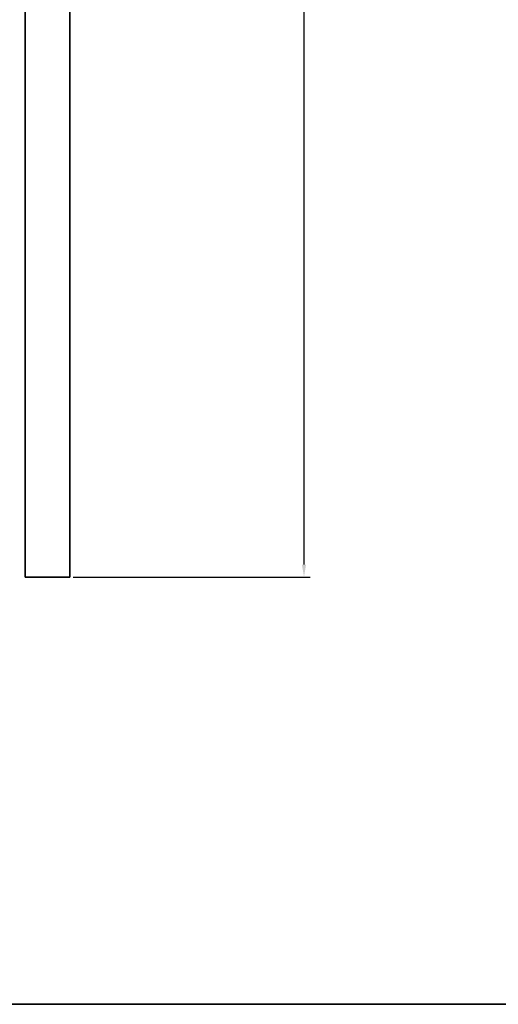
# Model space of a CAD drawing. Units: inches. Extents: x 1863 to 2938, y 1238 to 2492.
# Tile 5 of 12: x 2285 to 2381, y 1253 to 1452. Entities that reach past the tile are written whole.
import ezdxf

# ---------------------------------------------------------------- set-up
doc = ezdxf.new("R2010")
doc.units = ezdxf.units.IN
for name, color, linetype, lineweight in [('A-ANNO-DIMS', 2, 'Continuous', 18), ('A-ANNO-TTLB', 7, 'Continuous', 35), ('A-WALL', 7, 'Continuous', 35)]:
    doc.layers.add(name, color=color, linetype=linetype, lineweight=lineweight)
doc.styles.get("Standard").update_dxf_attribs({"font": 'arial.ttf'})
doc.dimstyles.new('ISO-25', dxfattribs={"dimtxt": 7, "dimasz": 2.5, "dimexe": 1.25, "dimexo": 0.625, "dimtad": 1, "dimdec": 0, "dimlunit": 3, "dimtxsty": 'Standard', "dimcen": 2.5, "dimadec": 0, "dimazin": 0, "dimtfac": 1, "dimtdec": 0, "dimtmove": 0, "dimatfit": 3, "dimfxl": 1, "dimarcsym": 0})

# ---------------------------------------------------------------- blocks, each defined once
blk = doc.blocks.new('*D3')
at = {"layer": 'A-ANNO-DIMS', "color": 0, "lineweight": -2, "transparency": 16777216}
for p, q in [((2295.26, 2076.56), (2343.03, 2076.56)), ((2341.78, 2074.06), (2341.78, 1342.06)), ((2295.26, 1339.56), (2343.03, 1339.56))]:
    blk.add_line(p, q, dxfattribs=at)
at = {"layer": 'A-ANNO-DIMS', "color": 0, "transparency": 16777216}
for points in [[(2341.36, 2074.06), (2342.2, 2074.06), (2341.78, 2076.56)], [(2341.36, 1342.06), (2342.2, 1342.06), (2341.78, 1339.56)]]:
    blk.add_solid(points, dxfattribs=at)
at = {"layer": 'Defpoints', "color": 0, "transparency": 16777216}
for p in [(2294.64, 2076.56), (2294.64, 1339.56), (2341.78, 1339.56)]:
    blk.add_point(p, dxfattribs=at)
at = {"layer": 'A-ANNO-DIMS', "color": 0, "transparency": 16777216, "insert": (2337.58, 1708.06), "char_height": 7, "attachment_point": 5, "rotation": 90}
blk.add_mtext('61\'-5"', dxfattribs=at)

msp = doc.modelspace()

# ---------------------------------------------------------------- linework, layer by layer
at = {"layer": 'A-ANNO-TTLB'}
msp.add_lwpolyline([(1863.2, 2492.19), (2938.41, 2492.19), (2938.41, 1253.47), (1863.2, 1253.47)], close=True, dxfattribs=at)
at = {"layer": 'A-WALL'}
for p, q in [((2285.64, 1339.56), (2285.64, 1495.56)), ((2294.64, 1495.56), (2294.64, 1339.56)), ((2294.64, 1339.56), (2285.64, 1339.56))]:
    msp.add_line(p, q, dxfattribs=at)

# ---------------------------------------------------------------- dimensions: what is measured, and where the dimension line sits
at = {"layer": 'A-ANNO-DIMS'}
dim = msp.add_linear_dim(base=(2341.78, 1339.56), p1=(2294.64, 2076.56), p2=(2294.64, 1339.56), angle=90, dimstyle='ISO-25', override={"dimclrd": 0, "dimclre": 0, "dimclrt": 0}, dxfattribs=at)
dim.commit()
dim.dimension.update_dxf_attribs({"geometry": '*D3', "text_midpoint": (2337.58, 1708.06)})

doc.saveas('drawing.dxf')
